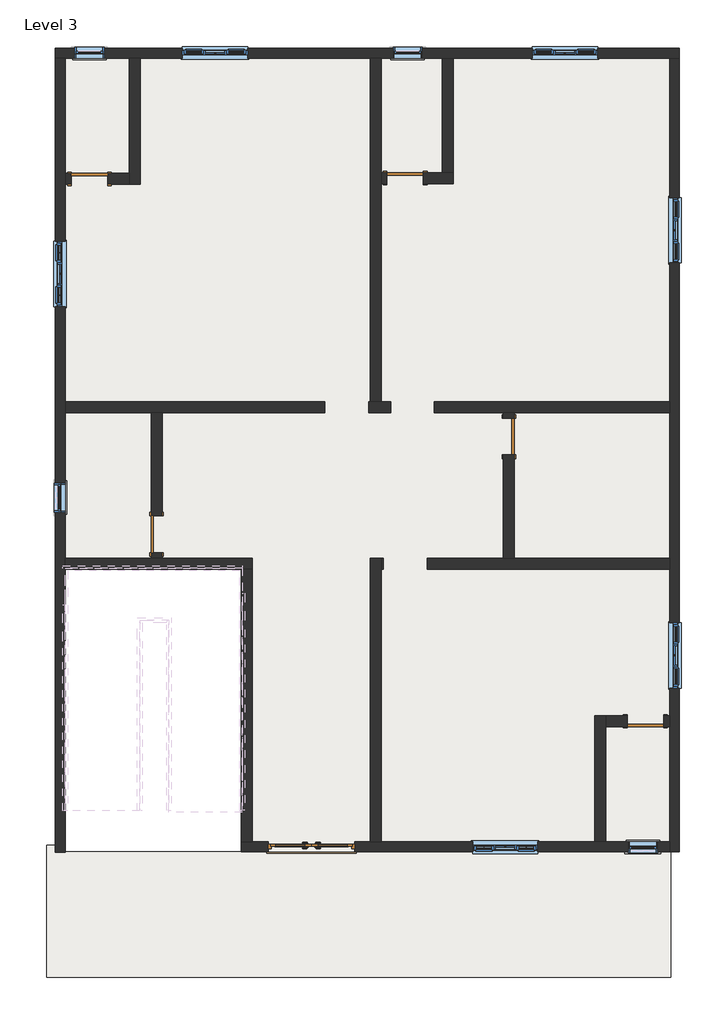
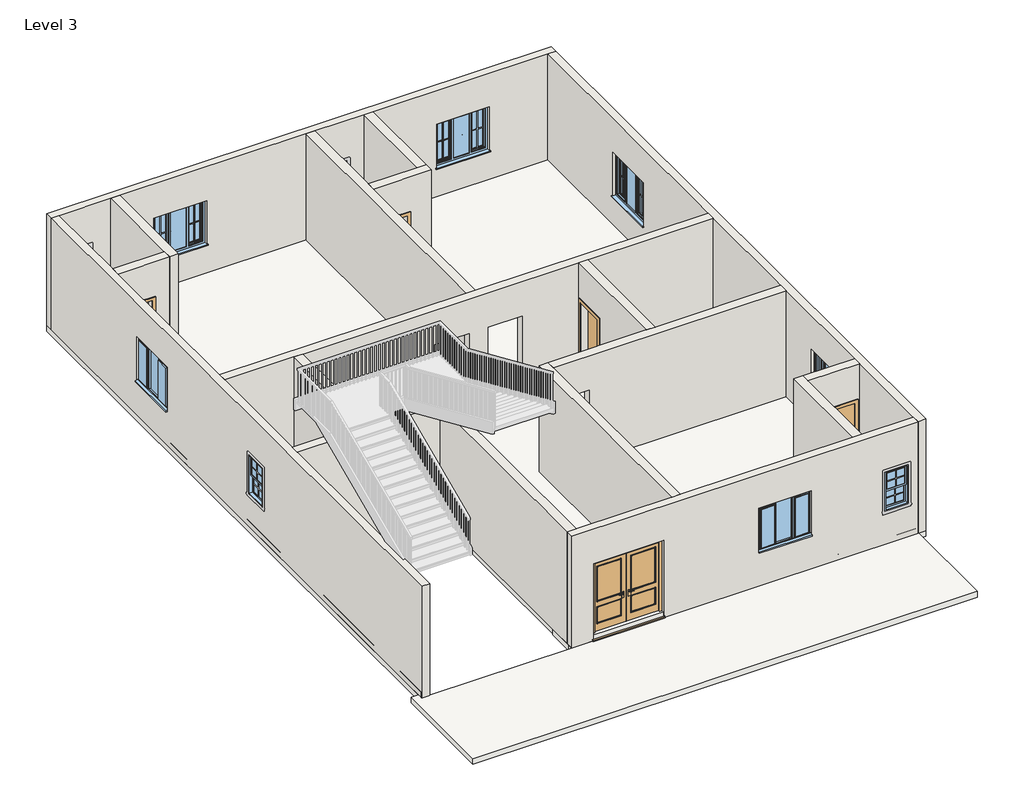
# One storey, part 1 of 6: 18 walls, 10 windows, 6 doors, 2 roofs, 2 slabs.
"""IFC4 building model written with IfcOpenShell, lengths in millimetres."""

from ifc_helpers import new_model, si_unit, frame, origin, place, context, project, spatial, polyline, outline, extrude, faceted_brep, transform, mapped, element, save
from components import doors_extdbl_2_1810x2110mm_9ab1935a, doors_extdbl_2_1810x2110mm_b7024f51, door_85036156, window_679d2811, windows_tpl_w_glazing_cross_bars_1360x1210mm_0306471f

model = new_model("IFC4")

# Units and contexts
model_context = context("Model", 3, world=origin())
ifc_project = project(units=[si_unit("LENGTHUNIT", "METRE", prefix="MILLI")], contexts=[model_context])

# Site, building, storey
site = spatial("IfcSite", under=ifc_project)
building = spatial("IfcBuilding", under=site)
storey = spatial("IfcBuildingStorey", under=building, Name="Level 3", Elevation=6096.0)

# Doors
placement = place(None, origin())
doors_extdbl_2_1810x2110mm_shape = doors_extdbl_2_1810x2110mm_9ab1935a(model_context)
doors_extdbl_2_1810x2110mm_2_shape = doors_extdbl_2_1810x2110mm_b7024f51(model_context)
element("IfcDoor", 1, ObjectType="Doors_ExtDbl_2 : 1810x2110mm", at=placement, inside=storey, context=model_context, shape_type="MappedRepresentation", body=[
    mapped(doors_extdbl_2_1810x2110mm_shape, transform((-2421.0852725, -7729.5064015, 6096.0), x_axis=(1.0, 0.0, 0.0), y_axis=(0.0, 1.0, 0.0), z_axis=(0.0, 0.0, 1.0))),
    mapped(doors_extdbl_2_1810x2110mm_2_shape, transform((-2421.0852725, -7729.5064015, 6096.0), x_axis=(1.0, 0.0, 0.0), y_axis=(0.0, 1.0, 0.0), z_axis=(0.0, 0.0, 1.0))),
])
door_shape = door_85036156(model_context)
element("IfcDoor", 2, ObjectType="Single-Flush : 30\" x 80\"", at=placement, inside=storey, context=model_context, shape_type="MappedRepresentation", body=[
    mapped(door_shape, transform((-7046.4415084, 6189.6935985, 6096.0), x_axis=(-1.0, 0.0, 0.0), y_axis=(0.0, -1.0, 0.0), z_axis=(0.0, 0.0, 1.0))),
])
element("IfcDoor", 3, ObjectType="Single-Flush : 30\" x 80\"", at=placement, inside=storey, context=model_context, shape_type="MappedRepresentation", body=[
    mapped(door_shape, transform((-467.8415084, 6203.2000968, 6096.0), x_axis=(-1.0, 0.0, 0.0), y_axis=(0.0, -1.0, 0.0), z_axis=(0.0, 0.0, 1.0))),
])
element("IfcDoor", 4, ObjectType="Single-Flush : 30\" x 80\"", at=placement, inside=storey, context=model_context, shape_type="MappedRepresentation", body=[
    mapped(door_shape, transform((-5649.4415084, -1217.2217109, 6096.0), x_axis=(0.0, -1.0, 0.0), y_axis=(1.0, 0.0, 0.0), z_axis=(0.0, 0.0, 1.0))),
])
element("IfcDoor", 5, ObjectType="Single-Flush : 30\" x 80\"", at=placement, inside=storey, context=model_context, shape_type="MappedRepresentation", body=[
    mapped(door_shape, transform((1691.1584916, 817.5935985, 6096.0), x_axis=(0.0, 1.0, 0.0), y_axis=(-1.0, 0.0, 0.0), z_axis=(0.0, 0.0, 1.0))),
])
element("IfcDoor", 6, ObjectType="Single-Flush : 30\" x 80\"", at=placement, inside=storey, context=model_context, shape_type="MappedRepresentation", body=[
    mapped(door_shape, transform((4535.9584916, -5113.3064015, 6096.0), x_axis=(1.0, 0.0, 0.0), y_axis=(0.0, 1.0, 0.0), z_axis=(0.0, 0.0, 1.0))),
])

# Roofs
element("IfcRoof", 7, ObjectType="Generic - 12\"", at=placement, inside=storey, context=model_context, shape_type="SweptSolid", body=[
    extrude(outline(polyline([(-7757.6415084, 8907.4935985), (5247.1584916, 8907.4935985), (5247.1584916, -7831.1064015), (-3879.0290366, -7831.1064015), (-3879.0290366, -6973.0610642), (-3866.3290366, -6973.0610642), (-3866.3290366, -1928.4217109), (-7554.4415084, -1928.4217109), (-7554.4415084, -7831.1064015), (-7757.6415084, -7831.1064015), (-7757.6415084, 8907.4935985)])), frame((0.0, 0.0, 6096.0), z_axis=(0.0, 0.0, 1.0), x_axis=(1.0, 0.0, 0.0)), (0.0, 0.0, 1.0), 152.4),
])
element("IfcRoof", 8, ObjectType="Generic - 12\"", at=placement, inside=storey, context=model_context, shape_type="SweptSolid", body=[
    extrude(outline(polyline([(-7757.6415084, 8907.4935985), (5247.1584916, 8907.4935985), (5247.1584916, -7831.1064015), (-3879.0290366, -7831.1064015), (-3879.0290366, -6973.0610642), (-3866.3290366, -6973.0610642), (-3866.3290366, -1928.4217109), (-7554.4415084, -1928.4217109), (-7554.4415084, -7831.1064015), (-7757.6415084, -7831.1064015), (-7757.6415084, 8907.4935985)])), frame((0.0, 0.0, 6096.0), z_axis=(0.0, 0.0, 1.0), x_axis=(1.0, 0.0, 0.0)), (0.0, 0.0, 1.0), 152.4),
])

# Slabs
element("IfcSlab", 9, ObjectType="Generic - 12\"", at=placement, inside=storey, context=model_context, shape_type="SweptSolid", body=[
    extrude(outline(polyline([(5247.1584916, 8907.4935985), (5247.1584916, -7831.1064015), (-3879.0290366, -7831.1064015), (-3879.0290366, -6973.0610642), (-3866.3290366, -6973.0610642), (-3866.3290366, -1928.4217109), (-7554.4415084, -1928.4217109), (-7554.4415084, -7831.1064015), (-7757.6415084, -7831.1064015), (-7757.6415084, 8907.4935985), (5247.1584916, 8907.4935985)])), frame((0.0, 0.0, 5943.6), z_axis=(0.0, 0.0, 1.0), x_axis=(1.0, 0.0, 0.0)), (0.0, 0.0, 1.0), 152.4),
])
element("IfcSlab", 10, ObjectType="Generic - 12\"", at=placement, inside=storey, context=model_context, shape_type="SweptSolid", body=[
    extrude(outline(polyline([(5063.8122085, -7701.6194881), (5063.8122085, -10451.1270757), (-7940.9877915, -10451.1270757), (-7940.9877915, -7701.6194881), (-7554.4415084, -7701.6194881), (-7554.4415084, -7831.1064015), (-3879.0290366, -7831.1064015), (-3879.0290366, -7701.6194881), (5063.8122085, -7701.6194881)])), frame((0.0, 0.0, 5943.6), z_axis=(0.0, 0.0, 1.0), x_axis=(1.0, 0.0, 0.0)), (0.0, 0.0, 1.0), 152.4),
])

# Walls
element("IfcWall", 11, ObjectType="Generic - 4.5\"", at=placement, inside=storey, context=model_context, shape_type="Brep", body=[
    faceted_brep([(-1232.0415084, 1312.8935985, 8206.0), (-1232.0415084, 1312.8935985, 6096.0), (-770.4415084, 1312.8935985, 6096.0), (-770.4415084, 1312.8935985, 8206.0), (139.5584916, 1312.8935985, 8206.0), (139.5584916, 1312.8935985, 6096.0), (1576.8584916, 1312.8935985, 6096.0), (1805.4584916, 1312.8935985, 6096.0), (5043.9584916, 1312.8935985, 6096.0), (5043.9584916, 1312.8935985, 9144.0), (1805.4584916, 1312.8935985, 9144.0), (1576.8584916, 1312.8935985, 9144.0), (-5535.1415084, 1312.8935985, 9144.0), (-5763.7415084, 1312.8935985, 9144.0), (-7554.4415084, 1312.8935985, 9144.0), (-7554.4415084, 1312.8935985, 6096.0), (-5763.7415084, 1312.8935985, 6096.0), (-5535.1415084, 1312.8935985, 6096.0), (-2142.0415084, 1312.8935985, 6096.0), (-2142.0415084, 1312.8935985, 8206.0), (-770.4415084, 1541.4935985, 6096.0), (-963.1415084, 1541.4935985, 6096.0), (-1191.7415084, 1541.4935985, 6096.0), (-1232.0415084, 1541.4935985, 6096.0), (-1232.0415084, 1541.4935985, 8206.0), (-2142.0415084, 1541.4935985, 8206.0), (-2142.0415084, 1541.4935985, 6096.0), (-7554.4415084, 1541.4935985, 6096.0), (-7554.4415084, 1541.4935985, 9144.0), (-1191.7415084, 1541.4935985, 9144.0), (-963.1415084, 1541.4935985, 9144.0), (5043.9584916, 1541.4935985, 9144.0), (5043.9584916, 1541.4935985, 6096.0), (139.5584916, 1541.4935985, 6096.0), (139.5584916, 1541.4935985, 8206.0), (-770.4415084, 1541.4935985, 8206.0)], [[[0, 1, 2, 3, 4, 5, 6, 7, 8, 9, 10, 11, 12, 13, 14, 15, 16, 17, 18, 19]], [[20, 21, 22, 23, 24, 25, 26, 27, 28, 29, 30, 31, 32, 33, 34, 35]], [[33, 32, 8, 7, 6, 5]], [[2, 1, 23, 22, 21, 20]], [[18, 17, 16, 15, 27, 26]], [[14, 13, 12, 11, 10, 9, 31, 30, 29, 28]], [[9, 8, 32, 31]], [[15, 14, 28, 27]], [[5, 4, 34, 33]], [[3, 2, 20, 35]], [[4, 3, 35, 34]], [[26, 25, 19, 18]], [[24, 23, 1, 0]], [[25, 24, 0, 19]]]),
])
element("IfcWall", 12, ObjectType="Generic - 4.5\"", at=placement, inside=storey, context=model_context, shape_type="Brep", body=[
    faceted_brep([(-1191.7415084, 8704.2935985, 6096.0), (-1191.7415084, 1541.4935985, 6096.0), (-1191.7415084, 1541.4935985, 9144.0), (-1191.7415084, 8704.2935985, 9144.0), (-963.1415084, 8704.2935985, 6096.0), (-963.1415084, 8704.2935985, 9144.0), (-963.1415084, 6317.5000968, 9144.0), (-963.1415084, 6088.9000968, 9144.0), (-963.1415084, 1541.4935985, 9144.0), (-963.1415084, 1541.4935985, 6096.0), (-963.1415084, 6088.9000968, 6096.0), (-963.1415084, 6317.5000968, 6096.0)], [[[0, 1, 2, 3]], [[4, 5, 6, 7, 8, 9, 10, 11]], [[1, 0, 4, 11, 10, 9]], [[3, 2, 8, 7, 6, 5]], [[0, 3, 5, 4]], [[2, 1, 9, 8]]]),
])
element("IfcWall", 13, ObjectType="Generic - 4.5\"", at=placement, inside=storey, context=model_context, shape_type="Brep", body=[
    faceted_brep([(-6220.9415084, 8704.2935985, 6096.0), (-6220.9415084, 6303.9935985, 6096.0), (-6220.9415084, 6075.3935985, 6096.0), (-6220.9415084, 6075.3935985, 9144.0), (-6220.9415084, 6303.9935985, 9144.0), (-6220.9415084, 8704.2935985, 9144.0), (-5992.3415084, 8704.2935985, 6096.0), (-5992.3415084, 8704.2935985, 9144.0), (-5992.3415084, 6075.3935985, 9144.0), (-5992.3415084, 6075.3935985, 6096.0)], [[[0, 1, 2, 3, 4, 5]], [[6, 7, 8, 9]], [[2, 1, 0, 6, 9]], [[5, 4, 3, 8, 7]], [[0, 5, 7, 6]], [[3, 2, 9, 8]]]),
])
element("IfcWall", 14, ObjectType="Generic - 4.5\"", at=placement, inside=storey, context=model_context, shape_type="SweptSolid", body=[
    extrude(outline(polyline([(6096.0, -7554.4415084), (6096.0, -7427.4415084), (8128.0, -7427.4415084), (8128.0, -6665.4415084), (6096.0, -6665.4415084), (6096.0, -6220.9415084), (9144.0, -6220.9415084), (9144.0, -7554.4415084), (6096.0, -7554.4415084)])), frame((0.0, 6075.3935985, 0.0), z_axis=(0.0, 1.0, 0.0), x_axis=(0.0, 0.0, 1.0)), (0.0, 0.0, 1.0), 228.6),
])
element("IfcWall", 15, ObjectType="Generic - 4.5\"", at=placement, inside=storey, context=model_context, shape_type="Brep", body=[
    faceted_brep([(-963.1415084, 6088.9000968, 6096.0), (-848.8415084, 6088.9000968, 6096.0), (-848.8415084, 6088.9000968, 8128.0), (-86.8415084, 6088.9000968, 8128.0), (-86.8415084, 6088.9000968, 6096.0), (535.4584916, 6088.9000968, 6096.0), (535.4584916, 6088.9000968, 9144.0), (-963.1415084, 6088.9000968, 9144.0), (-848.8415084, 6317.5000968, 8128.0), (-848.8415084, 6317.5000968, 6096.0), (-963.1415084, 6317.5000968, 6096.0), (-963.1415084, 6317.5000968, 9144.0), (306.8584916, 6317.5000968, 9144.0), (535.4584916, 6317.5000968, 9144.0), (535.4584916, 6317.5000968, 6096.0), (306.8584916, 6317.5000968, 6096.0), (-86.8415084, 6317.5000968, 6096.0), (-86.8415084, 6317.5000968, 8128.0)], [[[0, 1, 2, 3, 4, 5, 6, 7]], [[8, 9, 10, 11, 12, 13, 14, 15, 16, 17]], [[10, 9, 1, 0]], [[16, 15, 14, 5, 4]], [[7, 6, 13, 12, 11]], [[0, 7, 11, 10]], [[6, 5, 14, 13]], [[2, 1, 9, 8]], [[3, 2, 8, 17]], [[4, 3, 17, 16]]]),
])
element("IfcWall", 16, ObjectType="Generic - 4.5\"", at=placement, inside=storey, context=model_context, shape_type="SweptSolid", body=[
    extrude(outline(polyline([(535.4584916, 8704.2935985), (535.4584916, 6317.5000968), (306.8584916, 6317.5000968), (306.8584916, 8704.2935985), (535.4584916, 8704.2935985)])), frame((0.0, 0.0, 6096.0), z_axis=(0.0, 0.0, 1.0), x_axis=(1.0, 0.0, 0.0)), (0.0, 0.0, 1.0), 3048.0),
])
element("IfcWall", 17, ObjectType="Generic - 4.5\"", at=placement, inside=storey, context=model_context, shape_type="SweptSolid", body=[
    extrude(outline(polyline([(-1598.2217109, 8128.0), (-1598.2217109, 6096.0), (-1712.5217109, 6096.0), (-1712.5217109, 9144.0), (1312.8935985, 9144.0), (1312.8935985, 6096.0), (-836.2217109, 6096.0), (-836.2217109, 8128.0), (-1598.2217109, 8128.0)])), frame((-5763.7415084, 0.0, 0.0), z_axis=(1.0, 0.0, 0.0), x_axis=(0.0, 1.0, 0.0)), (0.0, 0.0, 1.0), 228.6),
])
element("IfcWall", 18, ObjectType="Generic - 4.5\"", at=placement, inside=storey, context=model_context, shape_type="Brep", body=[
    faceted_brep([(-7554.4415084, -1941.1217109, 6096.0), (-3879.0290366, -1941.1217109, 6096.0), (-3650.4290366, -1941.1217109, 6096.0), (-3650.4290366, -1941.1217109, 9144.0), (-3879.0290366, -1941.1217109, 9144.0), (-7554.4415084, -1941.1217109, 9144.0), (-7554.4415084, -1712.5217109, 6096.0), (-7554.4415084, -1712.5217109, 9144.0), (-5763.7415084, -1712.5217109, 9144.0), (-5535.1415084, -1712.5217109, 9144.0), (-3650.4290366, -1712.5217109, 9144.0), (-3650.4290366, -1712.5217109, 6096.0), (-5535.1415084, -1712.5217109, 6096.0), (-5763.7415084, -1712.5217109, 6096.0)], [[[0, 1, 2, 3, 4, 5]], [[6, 7, 8, 9, 10, 11, 12, 13]], [[2, 1, 0, 6, 13, 12, 11]], [[5, 4, 3, 10, 9, 8, 7]], [[0, 5, 7, 6]], [[3, 2, 11, 10]]]),
])
element("IfcWall", 19, ObjectType="Generic - 4.5\"", at=placement, inside=storey, context=model_context, shape_type="SweptSolid", body=[
    extrude(outline(polyline([(-3879.0290366, -7627.9064015), (-3879.0290366, -1941.1217109), (-3650.4290366, -1941.1217109), (-3650.4290366, -7627.9064015), (-3879.0290366, -7627.9064015)])), frame((0.0, 0.0, 6096.0), z_axis=(0.0, 0.0, 1.0), x_axis=(1.0, 0.0, 0.0)), (0.0, 0.0, 1.0), 3048.0),
])
element("IfcWall", 20, ObjectType="Generic - 4.5\"", at=placement, inside=storey, context=model_context, shape_type="SweptSolid", body=[
    extrude(outline(polyline([(1312.8935985, 6096.0), (1198.5935985, 6096.0), (1198.5935985, 8128.0), (436.5935985, 8128.0), (436.5935985, 6096.0), (-1712.5217109, 6096.0), (-1712.5217109, 9144.0), (1312.8935985, 9144.0), (1312.8935985, 6096.0)])), frame((1576.8584916, 0.0, 0.0), z_axis=(1.0, 0.0, 0.0), x_axis=(0.0, 1.0, 0.0)), (0.0, 0.0, 1.0), 228.6),
])
element("IfcWall", 21, ObjectType="Generic - 4.5\"", at=placement, inside=storey, context=model_context, shape_type="Brep", body=[
    faceted_brep([(-963.1415084, -7627.9064015, 6096.0), (-963.1415084, -1941.1217109, 6096.0), (-963.1415084, -1712.5217109, 6096.0), (-963.1415084, -1712.5217109, 9144.0), (-963.1415084, -1941.1217109, 9144.0), (-963.1415084, -7627.9064015, 9144.0), (-1191.7415084, -7627.9064015, 6096.0), (-1191.7415084, -7627.9064015, 9144.0), (-1191.7415084, -1712.5217109, 9144.0), (-1191.7415084, -1712.5217109, 6096.0)], [[[0, 1, 2, 3, 4, 5]], [[6, 7, 8, 9]], [[2, 1, 0, 6, 9]], [[5, 4, 3, 8, 7]], [[0, 5, 7, 6]], [[3, 2, 9, 8]]]),
])
element("IfcWall", 22, ObjectType="Generic - 4.5\"", at=placement, inside=storey, context=model_context, shape_type="Brep", body=[
    faceted_brep([(-922.8415084, -1712.5217109, 8206.0), (-922.8415084, -1712.5217109, 6096.0), (-963.1415084, -1712.5217109, 6096.0), (-963.1415084, -1712.5217109, 9144.0), (1576.8584916, -1712.5217109, 9144.0), (1805.4584916, -1712.5217109, 9144.0), (5043.9584916, -1712.5217109, 9144.0), (5043.9584916, -1712.5217109, 6096.0), (1805.4584916, -1712.5217109, 6096.0), (1576.8584916, -1712.5217109, 6096.0), (-12.8415084, -1712.5217109, 6096.0), (-12.8415084, -1712.5217109, 8206.0), (-963.1415084, -1941.1217109, 6096.0), (-922.8415084, -1941.1217109, 6096.0), (-922.8415084, -1941.1217109, 8206.0), (-12.8415084, -1941.1217109, 8206.0), (-12.8415084, -1941.1217109, 6096.0), (5043.9584916, -1941.1217109, 6096.0), (5043.9584916, -1941.1217109, 9144.0), (-963.1415084, -1941.1217109, 9144.0)], [[[0, 1, 2, 3, 4, 5, 6, 7, 8, 9, 10, 11]], [[12, 13, 14, 15, 16, 17, 18, 19]], [[2, 1, 13, 12]], [[10, 9, 8, 7, 17, 16]], [[6, 5, 4, 3, 19, 18]], [[3, 2, 12, 19]], [[7, 6, 18, 17]], [[16, 15, 11, 10]], [[14, 13, 1, 0]], [[15, 14, 0, 11]]]),
])
element("IfcWall", 23, ObjectType="Generic - 4.5\"", at=placement, inside=storey, context=model_context, shape_type="Brep", body=[
    faceted_brep([(3710.4584916, -7627.9064015, 6096.0), (3710.4584916, -5227.6064015, 6096.0), (3710.4584916, -4999.0064015, 6096.0), (3710.4584916, -4999.0064015, 9144.0), (3710.4584916, -5227.6064015, 9144.0), (3710.4584916, -7627.9064015, 9144.0), (3481.8584916, -7627.9064015, 6096.0), (3481.8584916, -7627.9064015, 9144.0), (3481.8584916, -4999.0064015, 9144.0), (3481.8584916, -4999.0064015, 6096.0)], [[[0, 1, 2, 3, 4, 5]], [[6, 7, 8, 9]], [[2, 1, 0, 6, 9]], [[5, 4, 3, 8, 7]], [[0, 5, 7, 6]], [[3, 2, 9, 8]]]),
])
element("IfcWall", 24, ObjectType="Generic - 4.5\"", at=placement, inside=storey, context=model_context, shape_type="SweptSolid", body=[
    extrude(outline(polyline([(8128.0, 4916.9584916), (6096.0, 4916.9584916), (6096.0, 5043.9584916), (9144.0, 5043.9584916), (9144.0, 3710.4584916), (6096.0, 3710.4584916), (6096.0, 4154.9584916), (8128.0, 4154.9584916), (8128.0, 4916.9584916)])), frame((0.0, -5227.6064015, 0.0), z_axis=(0.0, 1.0, 0.0), x_axis=(0.0, 0.0, 1.0)), (0.0, 0.0, 1.0), 228.6),
])
element("IfcWall", 25, ObjectType="Generic - 9\"", at=placement, inside=storey, context=model_context, shape_type="Brep", body=[
    faceted_brep([(-7757.6415084, 8704.2935985, 6096.0), (-7554.4415084, 8704.2935985, 6096.0), (-6220.9415084, 8704.2935985, 6096.0), (-5992.3415084, 8704.2935985, 6096.0), (-1191.7415084, 8704.2935985, 6096.0), (-963.1415084, 8704.2935985, 6096.0), (306.8584916, 8704.2935985, 6096.0), (535.4584916, 8704.2935985, 6096.0), (5043.9584916, 8704.2935985, 6096.0), (5247.1584916, 8704.2935985, 6096.0), (5247.1584916, 8704.2935985, 9144.0), (5043.9584916, 8704.2935985, 9144.0), (535.4584916, 8704.2935985, 9144.0), (306.8584916, 8704.2935985, 9144.0), (-963.1415084, 8704.2935985, 9144.0), (-1191.7415084, 8704.2935985, 9144.0), (-5992.3415084, 8704.2935985, 9144.0), (-6220.9415084, 8704.2935985, 9144.0), (-7554.4415084, 8704.2935985, 9144.0), (-7757.6415084, 8704.2935985, 9144.0), (2179.5584916, 8704.2935985, 8220.4), (3539.5584916, 8704.2935985, 8220.4), (3539.5584916, 8704.2935985, 7010.4), (2179.5584916, 8704.2935985, 7010.4), (-5110.2415084, 8704.2935985, 8220.4), (-3750.2415084, 8704.2935985, 8220.4), (-3750.2415084, 8704.2935985, 7010.4), (-5110.2415084, 8704.2935985, 7010.4), (-7351.2415084, 8704.2935985, 8077.2), (-6741.6415084, 8704.2935985, 8077.2), (-6741.6415084, 8704.2935985, 7010.4), (-7351.2415084, 8704.2935985, 7010.4), (-721.8415084, 8704.2935985, 8077.2), (-112.2415084, 8704.2935985, 8077.2), (-112.2415084, 8704.2935985, 7010.4), (-721.8415084, 8704.2935985, 7010.4), (-7757.6415084, 8907.4935985, 6096.0), (-7757.6415084, 8907.4935985, 9144.0), (5247.1584916, 8907.4935985, 9144.0), (5247.1584916, 8907.4935985, 6096.0), (2179.5584916, 8907.4935985, 8220.4), (2179.5584916, 8907.4935985, 7010.4), (3539.5584916, 8907.4935985, 7010.4), (3539.5584916, 8907.4935985, 8220.4), (-5110.2415084, 8907.4935985, 8220.4), (-5110.2415084, 8907.4935985, 7010.4), (-3750.2415084, 8907.4935985, 7010.4), (-3750.2415084, 8907.4935985, 8220.4), (-7351.2415084, 8907.4935985, 8077.2), (-7351.2415084, 8907.4935985, 7010.4), (-6741.6415084, 8907.4935985, 7010.4), (-6741.6415084, 8907.4935985, 8077.2), (-721.8415084, 8907.4935985, 8077.2), (-721.8415084, 8907.4935985, 7010.4), (-112.2415084, 8907.4935985, 7010.4), (-112.2415084, 8907.4935985, 8077.2)], [[[0, 1, 2, 3, 4, 5, 6, 7, 8, 9, 10, 11, 12, 13, 14, 15, 16, 17, 18, 19], [20, 21, 22, 23], [24, 25, 26, 27], [28, 29, 30, 31], [32, 33, 34, 35]], [[36, 37, 38, 39], [40, 41, 42, 43], [44, 45, 46, 47], [48, 49, 50, 51], [52, 53, 54, 55]], [[9, 8, 7, 6, 5, 4, 3, 2, 1, 0, 36, 39]], [[19, 18, 17, 16, 15, 14, 13, 12, 11, 10, 38, 37]], [[10, 9, 39, 38]], [[41, 40, 20, 23]], [[42, 41, 23, 22]], [[43, 42, 22, 21]], [[40, 43, 21, 20]], [[45, 44, 24, 27]], [[46, 45, 27, 26]], [[47, 46, 26, 25]], [[44, 47, 25, 24]], [[49, 48, 28, 31]], [[50, 49, 31, 30]], [[51, 50, 30, 29]], [[48, 51, 29, 28]], [[53, 52, 32, 35]], [[54, 53, 35, 34]], [[55, 54, 34, 33]], [[52, 55, 33, 32]], [[0, 19, 37, 36]]]),
])
element("IfcWall", 26, ObjectType="Generic - 9\"", at=placement, inside=storey, context=model_context, shape_type="Brep", body=[
    faceted_brep([(5043.9584916, 8704.2935985, 6096.0), (5043.9584916, 1541.4935985, 6096.0), (5043.9584916, 1312.8935985, 6096.0), (5043.9584916, -1712.5217109, 6096.0), (5043.9584916, -1941.1217109, 6096.0), (5043.9584916, -4999.0064015, 6096.0), (5043.9584916, -5227.6064015, 6096.0), (5043.9584916, -7627.9064015, 6096.0), (5043.9584916, -7831.1064015, 6096.0), (5043.9584916, -7831.1064015, 9144.0), (5043.9584916, -7627.9064015, 9144.0), (5043.9584916, -5227.6064015, 9144.0), (5043.9584916, -4999.0064015, 9144.0), (5043.9584916, -1941.1217109, 9144.0), (5043.9584916, -1712.5217109, 9144.0), (5043.9584916, 1312.8935985, 9144.0), (5043.9584916, 1541.4935985, 9144.0), (5043.9584916, 8704.2935985, 9144.0), (5043.9584916, 5796.5435985, 8220.4), (5043.9584916, 4436.5435985, 8220.4), (5043.9584916, 4436.5435985, 7010.4), (5043.9584916, 5796.5435985, 7010.4), (5043.9584916, -3061.7064015, 8220.4), (5043.9584916, -4421.7064015, 8220.4), (5043.9584916, -4421.7064015, 7010.4), (5043.9584916, -3061.7064015, 7010.4), (5247.1584916, 8704.2935985, 6096.0), (5247.1584916, 8704.2935985, 9144.0), (5247.1584916, -7831.1064015, 9144.0), (5247.1584916, -7831.1064015, 6096.0), (5247.1584916, 5796.5435985, 8220.4), (5247.1584916, 5796.5435985, 7010.4), (5247.1584916, 4436.5435985, 7010.4), (5247.1584916, 4436.5435985, 8220.4), (5247.1584916, -3061.7064015, 8220.4), (5247.1584916, -3061.7064015, 7010.4), (5247.1584916, -4421.7064015, 7010.4), (5247.1584916, -4421.7064015, 8220.4)], [[[0, 1, 2, 3, 4, 5, 6, 7, 8, 9, 10, 11, 12, 13, 14, 15, 16, 17], [18, 19, 20, 21], [22, 23, 24, 25]], [[26, 27, 28, 29], [30, 31, 32, 33], [34, 35, 36, 37]], [[8, 7, 6, 5, 4, 3, 2, 1, 0, 26, 29]], [[17, 16, 15, 14, 13, 12, 11, 10, 9, 28, 27]], [[31, 30, 18, 21]], [[32, 31, 21, 20]], [[33, 32, 20, 19]], [[30, 33, 19, 18]], [[35, 34, 22, 25]], [[36, 35, 25, 24]], [[37, 36, 24, 23]], [[34, 37, 23, 22]], [[0, 17, 27, 26]], [[9, 8, 29, 28]]]),
])
element("IfcWall", 27, ObjectType="Generic - 9\"", at=placement, inside=storey, context=model_context, shape_type="Brep", body=[
    faceted_brep([(5043.9584916, -7627.9064015, 6096.0), (3710.4584916, -7627.9064015, 6096.0), (3481.8584916, -7627.9064015, 6096.0), (-963.1415084, -7627.9064015, 6096.0), (-1191.7415084, -7627.9064015, 6096.0), (-1516.0852725, -7627.9064015, 6096.0), (-1516.0852725, -7627.9064015, 8206.0), (-3326.0852725, -7627.9064015, 8206.0), (-3326.0852725, -7627.9064015, 6096.0), (-3650.4290366, -7627.9064015, 6096.0), (-3879.0290366, -7627.9064015, 6096.0), (-3879.0290366, -7627.9064015, 9144.0), (-3650.4290366, -7627.9064015, 9144.0), (-1191.7415084, -7627.9064015, 9144.0), (-963.1415084, -7627.9064015, 9144.0), (3481.8584916, -7627.9064015, 9144.0), (3710.4584916, -7627.9064015, 9144.0), (5043.9584916, -7627.9064015, 9144.0), (2294.9584916, -7627.9064015, 8220.4), (934.9584916, -7627.9064015, 8220.4), (934.9584916, -7627.9064015, 7010.4), (2294.9584916, -7627.9064015, 7010.4), (4789.9584916, -7627.9064015, 8077.2), (4180.3584916, -7627.9064015, 8077.2), (4180.3584916, -7627.9064015, 7010.4), (4789.9584916, -7627.9064015, 7010.4), (-1516.0852725, -7831.1064015, 8206.0), (-1516.0852725, -7831.1064015, 6096.0), (5043.9584916, -7831.1064015, 6096.0), (5043.9584916, -7831.1064015, 9144.0), (-3879.0290366, -7831.1064015, 9144.0), (-3879.0290366, -7831.1064015, 6096.0), (-3326.0852725, -7831.1064015, 6096.0), (-3326.0852725, -7831.1064015, 8206.0), (2294.9584916, -7831.1064015, 8220.4), (2294.9584916, -7831.1064015, 7010.4), (934.9584916, -7831.1064015, 7010.4), (934.9584916, -7831.1064015, 8220.4), (4789.9584916, -7831.1064015, 8077.2), (4789.9584916, -7831.1064015, 7010.4), (4180.3584916, -7831.1064015, 7010.4), (4180.3584916, -7831.1064015, 8077.2)], [[[0, 1, 2, 3, 4, 5, 6, 7, 8, 9, 10, 11, 12, 13, 14, 15, 16, 17], [18, 19, 20, 21], [22, 23, 24, 25]], [[26, 27, 28, 29, 30, 31, 32, 33], [34, 35, 36, 37], [38, 39, 40, 41]], [[32, 31, 10, 9, 8]], [[28, 27, 5, 4, 3, 2, 1, 0]], [[17, 16, 15, 14, 13, 12, 11, 30, 29]], [[11, 10, 31, 30]], [[35, 34, 18, 21]], [[36, 35, 21, 20]], [[37, 36, 20, 19]], [[34, 37, 19, 18]], [[39, 38, 22, 25]], [[40, 39, 25, 24]], [[41, 40, 24, 23]], [[38, 41, 23, 22]], [[8, 7, 33, 32]], [[6, 5, 27, 26]], [[7, 6, 26, 33]], [[0, 17, 29, 28]]]),
])
element("IfcWall", 28, ObjectType="Generic - 9\"", at=placement, inside=storey, context=model_context, shape_type="Brep", body=[
    faceted_brep([(-7757.6415084, 8704.2935985, 6096.0), (-7757.6415084, -7843.8064015, 6096.0), (-7757.6415084, -7843.8064015, 9144.0), (-7757.6415084, 8704.2935985, 9144.0), (-7757.6415084, 3528.4935985, 8220.4), (-7757.6415084, 3528.4935985, 7010.4), (-7757.6415084, 4888.4935985, 7010.4), (-7757.6415084, 4888.4935985, 8220.4), (-7757.6415084, -760.0217109, 8077.2), (-7757.6415084, -760.0217109, 7010.4), (-7757.6415084, -150.4217109, 7010.4), (-7757.6415084, -150.4217109, 8077.2), (-7554.4415084, 8704.2935985, 6096.0), (-7554.4415084, 8704.2935985, 9144.0), (-7554.4415084, 6303.9935985, 9144.0), (-7554.4415084, 6075.3935985, 9144.0), (-7554.4415084, 1541.4935985, 9144.0), (-7554.4415084, 1312.8935985, 9144.0), (-7554.4415084, -1712.5217109, 9144.0), (-7554.4415084, -1941.1217109, 9144.0), (-7554.4415084, -7843.8064015, 9144.0), (-7554.4415084, -7843.8064015, 6096.0), (-7554.4415084, -1941.1217109, 6096.0), (-7554.4415084, -1712.5217109, 6096.0), (-7554.4415084, 1312.8935985, 6096.0), (-7554.4415084, 1541.4935985, 6096.0), (-7554.4415084, 6075.3935985, 6096.0), (-7554.4415084, 6303.9935985, 6096.0), (-7554.4415084, 3528.4935985, 8220.4), (-7554.4415084, 4888.4935985, 8220.4), (-7554.4415084, 4888.4935985, 7010.4), (-7554.4415084, 3528.4935985, 7010.4), (-7554.4415084, -760.0217109, 8077.2), (-7554.4415084, -150.4217109, 8077.2), (-7554.4415084, -150.4217109, 7010.4), (-7554.4415084, -760.0217109, 7010.4)], [[[0, 1, 2, 3], [4, 5, 6, 7], [8, 9, 10, 11]], [[12, 13, 14, 15, 16, 17, 18, 19, 20, 21, 22, 23, 24, 25, 26, 27], [28, 29, 30, 31], [32, 33, 34, 35]], [[1, 0, 12, 27, 26, 25, 24, 23, 22, 21]], [[2, 1, 21, 20]], [[3, 2, 20, 19, 18, 17, 16, 15, 14, 13]], [[5, 4, 28, 31]], [[6, 5, 31, 30]], [[7, 6, 30, 29]], [[4, 7, 29, 28]], [[9, 8, 32, 35]], [[10, 9, 35, 34]], [[11, 10, 34, 33]], [[8, 11, 33, 32]], [[0, 3, 13, 12]]]),
])

# Windows
window_shape = window_679d2811(model_context)
element("IfcWindow", 29, ObjectType="Window-Double-Hung : 24\" x 42\"", at=placement, inside=storey, context=model_context, shape_type="MappedRepresentation", body=[
    mapped(window_shape, transform((-7656.0415084, -455.2217109, 6096.0), x_axis=(0.0, 1.0, 0.0), y_axis=(-1.0, 0.0, 0.0), z_axis=(0.0, 0.0, 1.0))),
])
element("IfcWindow", 30, ObjectType="Window-Double-Hung : 24\" x 42\"", at=placement, inside=storey, context=model_context, shape_type="MappedRepresentation", body=[
    mapped(window_shape, transform((-7046.4415084, 8805.8935985, 6096.0), x_axis=(1.0, 0.0, 0.0), y_axis=(0.0, 1.0, 0.0), z_axis=(0.0, 0.0, 1.0))),
])
element("IfcWindow", 31, ObjectType="Window-Double-Hung : 24\" x 42\"", at=placement, inside=storey, context=model_context, shape_type="MappedRepresentation", body=[
    mapped(window_shape, transform((-417.0415084, 8805.8935985, 6096.0), x_axis=(1.0, 0.0, 0.0), y_axis=(0.0, 1.0, 0.0), z_axis=(0.0, 0.0, 1.0))),
])
element("IfcWindow", 32, ObjectType="Window-Double-Hung : 24\" x 42\"", at=placement, inside=storey, context=model_context, shape_type="MappedRepresentation", body=[
    mapped(window_shape, transform((4485.1584916, -7729.5064015, 6096.0), x_axis=(-1.0, 0.0, 0.0), y_axis=(0.0, -1.0, 0.0), z_axis=(0.0, 0.0, 1.0))),
])
windows_tpl_w_glazing_cross_bars_1360x1210mm_shape = windows_tpl_w_glazing_cross_bars_1360x1210mm_0306471f(model_context)
element("IfcWindow", 33, ObjectType="Windows_Tpl_w-Glazing_Cross-Bars : 1360x1210mm", at=placement, inside=storey, context=model_context, shape_type="MappedRepresentation", body=[
    mapped(windows_tpl_w_glazing_cross_bars_1360x1210mm_shape, transform((5137.1019238, 4614.8769318, 6110.4), x_axis=(0.0, -1.0, 0.0), y_axis=(1.0, 0.0, 0.0), z_axis=(0.0, 0.0, 1.0))),
])
element("IfcWindow", 34, ObjectType="Windows_Tpl_w-Glazing_Cross-Bars : 1360x1210mm", at=placement, inside=storey, context=model_context, shape_type="MappedRepresentation", body=[
    mapped(windows_tpl_w_glazing_cross_bars_1360x1210mm_shape, transform((5137.1019238, -4243.3730682, 6110.4), x_axis=(0.0, -1.0, 0.0), y_axis=(1.0, 0.0, 0.0), z_axis=(0.0, 0.0, 1.0))),
])
element("IfcWindow", 35, ObjectType="Windows_Tpl_w-Glazing_Cross-Bars : 1360x1210mm", at=placement, inside=storey, context=model_context, shape_type="MappedRepresentation", body=[
    mapped(windows_tpl_w_glazing_cross_bars_1360x1210mm_shape, transform((1113.2918249, -7721.0498337, 6110.4), x_axis=(-1.0, 0.0, 0.0), y_axis=(0.0, -1.0, 0.0), z_axis=(0.0, 0.0, 1.0))),
])
element("IfcWindow", 36, ObjectType="Windows_Tpl_w-Glazing_Cross-Bars : 1360x1210mm", at=placement, inside=storey, context=model_context, shape_type="MappedRepresentation", body=[
    mapped(windows_tpl_w_glazing_cross_bars_1360x1210mm_shape, transform((3361.2251583, 8797.4370307, 6110.4), x_axis=(1.0, 0.0, 0.0), y_axis=(0.0, 1.0, 0.0), z_axis=(0.0, 0.0, 1.0))),
])
element("IfcWindow", 37, ObjectType="Windows_Tpl_w-Glazing_Cross-Bars : 1360x1210mm", at=placement, inside=storey, context=model_context, shape_type="MappedRepresentation", body=[
    mapped(windows_tpl_w_glazing_cross_bars_1360x1210mm_shape, transform((-3928.5748417, 8797.4370307, 6110.4), x_axis=(1.0, 0.0, 0.0), y_axis=(0.0, 1.0, 0.0), z_axis=(0.0, 0.0, 1.0))),
])
element("IfcWindow", 38, ObjectType="Windows_Tpl_w-Glazing_Cross-Bars : 1360x1210mm", at=placement, inside=storey, context=model_context, shape_type="MappedRepresentation", body=[
    mapped(windows_tpl_w_glazing_cross_bars_1360x1210mm_shape, transform((-7647.5849406, 4710.1602652, 6110.4), x_axis=(0.0, 1.0, 0.0), y_axis=(-1.0, 0.0, 0.0), z_axis=(0.0, 0.0, 1.0))),
])

save(model, "model.ifc")

# Revit data of these elements
# Type "Doors_ExtDbl_2 : 1810x2110mm"
#   Type Mark = "8"
#   Type Comments = "External Double"
#   Operation = "DoubleDoorSingleSwing"
#   Construction Type Id = "GSP4R"
#   Keynote = "L20"
#   Analytic Construction = "1/8 in Pilkington single glazing"
#   Wrap Layers (Int) from Ext = 0' - 6.98819"
#   Wrap Layers (Ext) from Ext = 0' - 4.03543"
#   Visual Light Transmittance = 0.9
#   Top of Lock Rail = 2' - 11.43307"
#   Thickness = 0' - 1.73228"
#   Stile Shutting = 0' - 4.92126"
#   Stile - Top Rail = 0' - 5.90551"
#   Stile - Lock Rail = 0' - 5.90551"
#   Stile - Hanging = 0' - 3.93701"
#   Stile - Bottom Rail = 0' - 11.81102"
#   Solar Heat Gain Coefficient = 0.78
#   Rough Width = 5' - 11.25984"
#   Rough Height = 6' - 11.07087"
#   O/A Frame Width = 0' - 2.51969"
#   Heat Transfer Coefficient (U) = 0.6496 BTU/(h·ft²·°F)
#   Handle Z Distance = 3' - 1.40157"
#   Glazing Thickness = 0' - 0.94488"
#   FrameWidth = 0' - 1.65354"
#   FrameOffset - External = 0' - 2.55906"
#   FrameDepth = 0' - 3.50394"
#   Door Panel Width = 2' - 9.54331"
#   Door Panel Thickness = 0' - 1.73228"
#   Door Panel Height = 6' - 6.74016"
#   Cill Thickness = 0' - 2.14567"
#   Cill Projection = 0' - 1.1811"
#   Handle X Distance = 0' - 2.95276"
#   Height = 6' - 11.07087"
#   Structural Tolerance = 0' - 0.25591"
#   Tolerance = 0' - 0.11811"
#   Undercut = 0' - 0.15748"
#   Width = 5' - 11.25984"
#   Cill Extension = 0' - 0.98425"
#   Cavity Closer Width = 0' - 1.9685"
#   Cavity Closer Offset from Ext = 0' - 4.03543"
#   Cavity Closer Depth = 0' - 3.34646"
#   Vis - Ironmongery = yes
#   Vis - Cavity Closers = yes
#   Define Thermal Properties by = 1
#   Function = 1
#   Material Glass = Door - Glazing
#   Handle Style = element 387460
#   Material Door = Door - Panel
#   Material Frame = Door - Frame/Mullion
#   Material Ironmongery = Door - Handle
#   Wall Closure = (empty or 0)
# Type "Single-Flush : 30\" x 80\""
#   Type Mark = "5"
#   Construction Type Id = "MDOOR"
#   Assembly Code = "C1020"
#   Analytic Construction = "Metal"
#   Thickness = 0' - 2"
#   Heat Transfer Coefficient (U) = 0.651978 BTU/(h·ft²·°F)
#   Height = 6' - 8"
#   Trim Projection Ext = 0' - 1"
#   Trim Projection Int = 0' - 1"
#   Trim Width = 0' - 3"
#   Width = 2' - 6"
#   Define Thermal Properties by = 1
#   Define Thermal Properties by = 1
#   Door Material = Door - Panel
#   Frame Material = Door - Frame
#   Visual Light Transmittance = 0
#   Solar Heat Gain Coefficient = 0
#   Function = (empty or 0)
#   Wall Closure = (empty or 0)
# Type "Generic - 12\""
#   Assembly Code = "B1020"
#   Layers, outside or top first: 0' - 6" no material (function 1)
# Type "Generic - 12\""
#   Assembly Code = "B1010"
#   Function = 0
#   Layers, outside or top first: 0' - 6" no material (function 1)
# Type "Generic - 4.5\""
#   Assembly Code = "B2010"
#   Layers, outside or top first: 0' - 9" no material (function 1)
# Type "Generic - 9\""
#   Assembly Code = "B2010"
#   Layers, outside or top first: 0' - 8" no material (function 1)
# Type "Window-Double-Hung : 24\" x 42\""
#   Type Mark = "10"
#   Fire Rating = "0.5h"
#   Construction Type Id = "DG-DR"
#   Assembly Code = "B2020100"
#   Analytic Construction = "Double glazing - domestic"
#   Wall Thickness [instance default] = 0' - 6"
#   Window Inset [instance default] = 0' - 0"
#   Visual Light Transmittance = 0.81
#   Thermal Resistance (R) = 1.8146 (h·ft²·°F)/BTU
#   Solar Heat Gain Coefficient = 0.76
#   Muntin Width = 1' - 6"
#   Muntin Height = 1' - 5 1/8"
#   Interior Wall Closure [instance default] = 0' - 1 1/2"
#   Rough Width = 2' - 0 1/2"
#   Rough Height = 3' - 6 1/2"
#   Frame Extension [instance default] = 0' - 1 1/4"
#   Exterior Wall Closure [instance default] = 0' - 0 1/2"
#   Extension Jamb [instance default] = 0' - 1 1/2"
#   Heat Transfer Coefficient (U) = 0.5511 BTU/(h·ft²·°F)
#   Height = 3' - 6"
#   Width = 2' - 0"
#   Define Thermal Properties by = 1
#   Top Muntin Visibility = yes
#   Indicator Visibility [instance default] = yes
#   Extension Jamb Visibility [instance default] = yes
#   Interior Trim Visibility [instance default] = yes
#   Exterior Trim Visibility [instance default] = yes
#   Define Thermal Properties by = 1
#   Bottom Muntin Visibility = yes
#   Muntin Pattern = Muntin Pattern_2x2 : Muntin Pattern_2x2
#   Interior Trim Material = Wood - Stained
#   Interior Trim = Trim-Window-Interior-Flat : Picture Frame
#   Exterior Trim Material = Clad - White
#   Exterior Trim = Trim-Window-Exterior-Flat : with Sill
#   Glass Panel Material = Glass
#   Exterior Frame Material = Clad - White
#   Interior Frame Material = Wood - Stained
#   Wall Closure = (empty or 0)
# Type "Windows_Tpl_w-Glazing_Cross-Bars : 1360x1210mm"
#   Type Mark = "21"
#   Operation = "TriplePanelVertical"
#   Construction Type Id = "GSP4R"
#   Manufacturer = "Revit"
#   Keynote = "L10"
#   Analytic Construction = "1/8 in Pilkington single glazing"
#   Wrap Layers (Ext) from Ext = 0' - 4.03543"
#   Wrap Layers (Int) from Ext = 0' - 6.98819"
#   Window Board Projection = 0' - 0.98425"
#   Window Board Extension = 0' - 0.98425"
#   Visual Light Transmittance = 0.9
#   Solar Heat Gain Coefficient = 0.78
#   Rough Width = 4' - 5.54331"
#   Rough Height = 3' - 11.6378"
#   Height = 3' - 11.6378"
#   Width = 4' - 5.54331"
#   Heat Transfer Coefficient (U) = 0.6496 BTU/(h·ft²·°F)
#   Glazing Thickness = 0' - 0.94488"
#   Glazing Bar Thickness = 0' - 0.7874"
#   FrameOffset - External = 0' - 1.9685"
#   Frame Depth = 0' - 2.55906"
#   Default Head Height = 6' - 11.07087"
#   Cill Depth = 0' - 3.44488"
#   Cavity Closer Width = 0' - 1.9685"
#   Cavity Closer Offset from Ext = 0' - 4.03543"
#   Cavity Closer Depth = 0' - 3.34646"
#   Vis - Glazing Bars = yes
#   Vis - Cavity Closers = yes
#   Define Thermal Properties by = 1
#   Material Trim = Window Frame
#   Material Glazing Bars = Window Frame
#   Material Glass = Glass
#   Material Frame = Window Frame
#   Wall Closure = (empty or 0)
# Element 1 (IfcDoor, "Doors_ExtDbl_2 : 1810x2110mm")
#   Phase Created = New Construction
#   Materials on its faces: "Door - Panel", "Door - Handle", "Door - Frame/Mullion", "Door - Glazing"
# Elements 2, 3, 4, 5, 6 (IfcDoor, "Single-Flush : 30\" x 80\"")
#   Phase Created = New Construction
#   Materials on its faces: "Door - Frame", "Door - Panel"
# Elements 7, 8 (IfcRoof, "Generic - 12\"")
#   built-in parameter 1001705 = 20.5 (stored number, unit not read)
#   built-in parameter 1001710 = 33615
#   Phase Created = New Construction
#   Materials on its faces: "Default Roof"
# Element 9 (IfcSlab, "Generic - 12\"")
#   Height Offset From Level = 0' - 0"
#   Phase Created = New Construction
#   Materials on its faces: "Default Floor"
# Element 10 (IfcSlab, "Generic - 12\"")
#   Height Offset From Level = 0' - 0"
#   Phase Created = New Construction
#   Materials on its faces: "Default Floor", "Concrete, Precast", "Default Mass Interior Wall"
# Elements 11, 12, 13, 14, 15, 16, 17, 20, 21, 22, 23, 24 (IfcWall, "Generic - 4.5\"")
#   Top Offset = 0' - 0"
#   Base Offset = 0' - 0"
#   wall height = 10' - 0"
#   Phase Created = New Construction
#   Base Constraint = Level 3
#   Top Constraint = Level 4
#   Materials on its faces: "Default Wall"
# Element 18 (IfcWall, "Generic - 4.5\"")
#   Top Offset = 0' - 0"
#   Base Offset = 0' - 0"
#   wall height = 10' - 0"
#   Phase Created = New Construction
#   Base Constraint = Level 3
#   Top Constraint = Level 4
#   Materials on its faces: "Default Wall", "Concrete, Precast"
# Element 19 (IfcWall, "Generic - 4.5\"")
#   Top Offset = 0' - 0"
#   Base Offset = 0' - 0"
#   wall height = 10' - 0"
#   Phase Created = New Construction
#   Base Constraint = Level 3
#   Top Constraint = Level 4
#   Materials on its faces: "Default Wall", "Bed-white fabric"
# Elements 25, 28 (IfcWall, "Generic - 9\"")
#   Top Offset = 0' - 0"
#   Base Offset = 0' - 0"
#   wall height = 10' - 0"
#   Phase Created = New Construction
#   Base Constraint = Level 3
#   Top Constraint = Level 4
#   Materials on its faces: "Default Wall", "Bed-white fabric"
# Element 26 (IfcWall, "Generic - 9\"")
#   Top Offset = 0' - 0"
#   Base Offset = 0' - 0"
#   wall height = 10' - 0"
#   Phase Created = New Construction
#   Base Constraint = Level 3
#   Top Constraint = Level 4
#   Materials on its faces: "Default Wall", "Bed-white fabric", "Bed-red fabric"
# Element 27 (IfcWall, "Generic - 9\"")
#   Top Offset = 0' - 0"
#   Base Offset = 0' - 0"
#   wall height = 10' - 0"
#   Phase Created = New Construction
#   Base Constraint = Level 3
#   Top Constraint = Level 4
#   Materials on its faces: "Default Wall", "Bed-red fabric", "Bed-white fabric"
# Element 29 (IfcWindow, "Window-Double-Hung : 24\" x 42\"")
#   Mark = "34"
#   Window Inset = 0' - 0"
#   Interior Wall Closure = 0' - 1 1/2"
#   Frame Extension = 0' - 1 1/4"
#   Exterior Wall Closure = 0' - 0 1/2"
#   Interior Trim Visibility = yes
#   Indicator Visibility = yes
#   Exterior Trim Visibility = yes
#   Phase Created = New Construction
#   Materials on its faces: "Wood - Stained", "Glass", "Clad - White"
# Element 30 (IfcWindow, "Window-Double-Hung : 24\" x 42\"")
#   Mark = "35"
#   Window Inset = 0' - 0"
#   Interior Wall Closure = 0' - 1 1/2"
#   Frame Extension = 0' - 1 1/4"
#   Exterior Wall Closure = 0' - 0 1/2"
#   Interior Trim Visibility = yes
#   Indicator Visibility = yes
#   Exterior Trim Visibility = yes
#   Phase Created = New Construction
#   Materials on its faces: "Wood - Stained", "Glass", "Clad - White"
# Element 31 (IfcWindow, "Window-Double-Hung : 24\" x 42\"")
#   Mark = "36"
#   Window Inset = 0' - 0"
#   Interior Wall Closure = 0' - 1 1/2"
#   Frame Extension = 0' - 1 1/4"
#   Exterior Wall Closure = 0' - 0 1/2"
#   Interior Trim Visibility = yes
#   Indicator Visibility = yes
#   Exterior Trim Visibility = yes
#   Phase Created = New Construction
#   Materials on its faces: "Wood - Stained", "Glass", "Clad - White"
# Element 32 (IfcWindow, "Window-Double-Hung : 24\" x 42\"")
#   Mark = "37"
#   Window Inset = 0' - 0"
#   Interior Wall Closure = 0' - 1 1/2"
#   Frame Extension = 0' - 1 1/4"
#   Exterior Wall Closure = 0' - 0 1/2"
#   Interior Trim Visibility = yes
#   Indicator Visibility = yes
#   Exterior Trim Visibility = yes
#   Phase Created = New Construction
#   Materials on its faces: "Wood - Stained", "Glass", "Clad - White"
# Element 33 (IfcWindow, "Windows_Tpl_w-Glazing_Cross-Bars : 1360x1210mm")
#   Mark = "28"
#   Phase Created = New Construction
#   Materials on its faces: "Window Frame", "Glass"
# Element 34 (IfcWindow, "Windows_Tpl_w-Glazing_Cross-Bars : 1360x1210mm")
#   Mark = "29"
#   Phase Created = New Construction
#   Materials on its faces: "Window Frame", "Glass"
# Element 35 (IfcWindow, "Windows_Tpl_w-Glazing_Cross-Bars : 1360x1210mm")
#   Mark = "30"
#   Phase Created = New Construction
#   Materials on its faces: "Window Frame", "Glass"
# Element 36 (IfcWindow, "Windows_Tpl_w-Glazing_Cross-Bars : 1360x1210mm")
#   Mark = "31"
#   Phase Created = New Construction
#   Materials on its faces: "Window Frame", "Glass"
# Element 37 (IfcWindow, "Windows_Tpl_w-Glazing_Cross-Bars : 1360x1210mm")
#   Mark = "32"
#   Phase Created = New Construction
#   Materials on its faces: "Window Frame", "Glass"
# Element 38 (IfcWindow, "Windows_Tpl_w-Glazing_Cross-Bars : 1360x1210mm")
#   Mark = "33"
#   Phase Created = New Construction
#   Materials on its faces: "Window Frame", "Glass"
# Materials
#   "Door - Glazing": colour RGB 0 0 255, transparency 0.75
#   "Door - Panel": class "Wood", colour RGB 210 159 95, transparency 0, Cost = 0
#   "Door - Frame/Mullion": class "Wood", colour RGB 212 179 113, transparency 0
#   "Door - Handle": colour RGB 247 247 247, transparency 0
#   "Door - Frame": colour RGB 118 70 51, transparency 0, Cost = 0
#   "Wood - Stained": class "Wood", colour RGB 224 178 126, transparency 0, Cost = 0
#   "Clad - White": class "Wood", colour RGB 242 242 238, transparency 0, Cost = 0
#   "Glass": class "Glass", colour RGB 0 128 192, transparency 0.75, Description = "Soda Lime Glass", Cost = 0
#   "Window Frame": colour RGB 249 249 249, transparency 0
#   "Default Roof": colour RGB 88 101 114, transparency 0, Cost = 0
#   "Default Floor": colour RGB 128 128 128, transparency 0, Cost = 0
#   "Concrete, Precast": class "Concrete", colour RGB 198 187 187, transparency 0, Description = "Precast concrete", Cost = 0
#   "Default Mass Interior Wall": class "Generic", colour RGB 195 229 126, transparency 0, Cost = 0
#   "Default Wall": colour RGB 128 128 128, transparency 0, Cost = 0
#   "Bed-white fabric": class "Paint", colour RGB 220 220 220, transparency 0
#   "Bed-red fabric": class "Fabric", colour RGB 76 38 38, transparency 0
